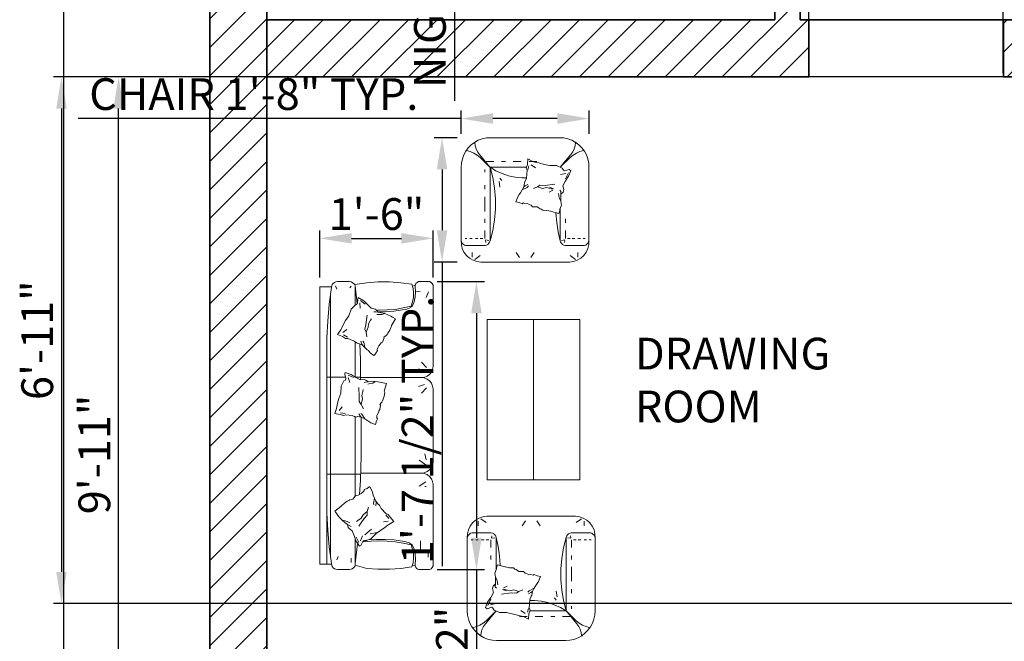
# Model space of a CAD drawing. Units: inches. Extents: x -33 to 381, y -443 to 47.
# Tile 2 of 5: x -33 to 122, y -308 to -210. Entities that reach past the tile are written whole.
import ezdxf

# ---------------------------------------------------------------- set-up
doc = ezdxf.new("R2010")
doc.units = ezdxf.units.IN
for name, color, linetype, lineweight in [('A-ANNO-DIMS', 2, 'Continuous', 18), ('A-AREA-IDEN', 7, 'Continuous', 18), ('A-WALL', 7, 'Continuous', 35), ('A-WALL-PATT', 251, 'Continuous', 13), ('furn', 8, 'Continuous', 13)]:
    doc.layers.add(name, color=color, linetype=linetype, lineweight=lineweight)
doc.styles.get("Standard").update_dxf_attribs({"font": 'arial.ttf'})
doc.dimstyles.new('ISO-25', dxfattribs={"dimtxt": 5, "dimasz": 5, "dimexe": 1.25, "dimexo": 0.625, "dimtad": 1, "dimlunit": 3, "dimtxsty": 'Standard', "dimcen": 2.5, "dimadec": 0, "dimazin": 0, "dimtfac": 1, "dimtmove": 0, "dimatfit": 3, "dimfxl": 1, "dimarcsym": 0})

# ---------------------------------------------------------------- blocks, each defined once
blk = doc.blocks.new('sofa-43')
at = {"color": 0, "linetype": 'ByBlock'}
for p, q in [((-0.038, 0.929), (-0.045, 0.917)), ((-0.045, 0.917), (-0.038, 0.929)), ((-0.045, 0.917), (-0.045, 0.824)), ((-0.045, 0.917), (-0.045, 0.824)), ((-0.028, 0.939), (-0.038, 0.929)), ((-0.038, 0.929), (-0.028, 0.939)), ((-0.015, 0.947), (-0.028, 0.939)), ((-0.028, 0.939), (-0.015, 0.947)), ((-0.003, 0.947), (-0.015, 0.947)), ((-0.015, 0.947), (-0.003, 0.947)), ((0.665, 0.947), (-0.003, 0.947)), ((-0.003, 0.947), (0.665, 0.947)), ((0.042, 0.909), (0.087, 0.889)), ((0.687, 0.942), (0.665, 0.947)), ((0.687, 0.942), (0.665, 0.947)), ((0.712, 0.932), (0.687, 0.942)), ((0.712, 0.932), (0.687, 0.942)), ((0.73, 0.917), (0.712, 0.932)), ((0.73, 0.917), (0.712, 0.932)), ((0.745, 0.897), (0.73, 0.917)), ((0.745, 0.897), (0.73, 0.917)), ((0.785, 0.917), (0.77, 0.897)), ((0.77, 0.897), (0.785, 0.917)), ((0.802, 0.932), (0.785, 0.917)), ((0.785, 0.917), (0.802, 0.932)), ((0.827, 0.942), (0.802, 0.932)), ((0.802, 0.932), (0.827, 0.942)), ((0.85, 0.947), (0.827, 0.942)), ((0.827, 0.942), (0.85, 0.947)), ((1.462, 0.947), (0.85, 0.947)), ((0.85, 0.947), (1.462, 0.947)), ((1.487, 0.942), (1.462, 0.947)), ((1.487, 0.942), (1.462, 0.947)), ((1.509, 0.932), (1.487, 0.942)), ((1.509, 0.932), (1.487, 0.942)), ((1.527, 0.917), (1.509, 0.932)), ((1.527, 0.917), (1.509, 0.932)), ((1.542, 0.897), (1.527, 0.917)), ((1.542, 0.897), (1.527, 0.917)), ((1.582, 0.917), (1.567, 0.897)), ((1.567, 0.897), (1.582, 0.917)), ((1.602, 0.932), (1.582, 0.917)), ((1.582, 0.917), (1.602, 0.932)), ((1.624, 0.942), (1.602, 0.932)), ((1.602, 0.932), (1.624, 0.942)), ((1.647, 0.947), (1.624, 0.942)), ((1.624, 0.942), (1.647, 0.947)), ((2.317, 0.947), (1.647, 0.947)), ((1.647, 0.947), (2.317, 0.947)), ((2.257, 0.904), (2.207, 0.904)), ((2.329, 0.947), (2.317, 0.947)), ((2.329, 0.947), (2.317, 0.947)), ((2.342, 0.939), (2.329, 0.947)), ((2.342, 0.939), (2.329, 0.947)), ((2.352, 0.929), (2.342, 0.939)), ((2.352, 0.929), (2.342, 0.939)), ((2.359, 0.917), (2.352, 0.929)), ((2.359, 0.917), (2.352, 0.929)), ((2.359, 0.824), (2.359, 0.917)), ((2.359, 0.917), (2.359, 0.824)), ((-0.045, 0.824), (-0.038, 0.812)), ((-0.045, 0.824), (-0.038, 0.812)), ((0.04, 0.799), (0.037, 0.839)), ((0.672, 0.892), (0.627, 0.849)), ((0.7, 0.874), (0.685, 0.824)), ((0.755, 0.872), (0.745, 0.897)), ((0.755, 0.872), (0.745, 0.897)), ((0.757, 0.849), (0.755, 0.872)), ((0.757, 0.849), (0.755, 0.872)), ((0.76, 0.872), (0.757, 0.849)), ((0.757, 0.849), (0.76, 0.872)), ((0.757, 0.345), (0.757, 0.849)), ((0.77, 0.897), (0.76, 0.872)), ((0.76, 0.872), (0.77, 0.897)), ((0.815, 0.874), (0.83, 0.824)), ((0.842, 0.892), (0.887, 0.849)), ((1.442, 0.887), (1.394, 0.877)), ((1.484, 0.884), (1.447, 0.829)), ((1.552, 0.872), (1.542, 0.897)), ((1.552, 0.872), (1.542, 0.897)), ((1.554, 0.849), (1.552, 0.872)), ((1.554, 0.849), (1.552, 0.872)), ((1.557, 0.872), (1.554, 0.849)), ((1.554, 0.849), (1.557, 0.872)), ((1.554, 0.345), (1.554, 0.849)), ((1.567, 0.897), (1.557, 0.872)), ((1.557, 0.872), (1.567, 0.897)), ((1.627, 0.884), (1.664, 0.829)), ((1.667, 0.887), (1.667, 0.877)), ((2.194, 0.842), (2.119, 0.842)), ((2.352, 0.812), (2.359, 0.824)), ((2.359, 0.824), (2.352, 0.812)), ((-0.038, 0.812), (-0.028, 0.802)), ((-0.038, 0.812), (-0.028, 0.802)), ((-0.023, 0.769), (-0.035, 0.677)), ((-0.023, 0.769), (-0.035, 0.677)), ((-0.028, 0.802), (-0.015, 0.797)), ((-0.028, 0.802), (-0.015, 0.797)), ((0.012, 0.779), (-0.023, 0.769)), ((-0.0064, 0.7737), (-0.023, 0.769)), ((-0.015, 0.797), (-0.0064, 0.7737)), ((-0.015, 0.797), (-0.003, 0.797)), ((-0.0064, 0.7737), (-0.015, 0.797)), ((0.04, 0.799), (-0.003, 0.797)), ((0.05, 0.782), (0.012, 0.779)), ((0.082, 0.797), (0.04, 0.799)), ((0.087, 0.782), (0.05, 0.782)), ((0.125, 0.787), (0.082, 0.797)), ((0.125, 0.774), (0.087, 0.782)), ((0.162, 0.772), (0.125, 0.787)), ((0.16, 0.762), (0.125, 0.774)), ((0.175, 0.697), (0.16, 0.762)), ((0.177, 0.747), (0.162, 0.772)), ((0.187, 0.719), (0.177, 0.747)), ((2.127, 0.719), (2.137, 0.747)), ((2.137, 0.747), (2.152, 0.772)), ((2.139, 0.697), (2.154, 0.762)), ((2.152, 0.772), (2.189, 0.787)), ((2.154, 0.762), (2.189, 0.774)), ((2.189, 0.787), (2.232, 0.797)), ((2.189, 0.774), (2.227, 0.782)), ((2.227, 0.782), (2.264, 0.782)), ((2.232, 0.797), (2.274, 0.799)), ((2.264, 0.782), (2.302, 0.779)), ((2.274, 0.799), (2.317, 0.797)), ((2.302, 0.779), (2.337, 0.769)), ((2.329, 0.797), (2.317, 0.797)), ((2.3218, 0.7734), (2.329, 0.797)), ((2.3218, 0.7734), (2.329, 0.797)), ((2.337, 0.769), (2.3218, 0.7734)), ((2.329, 0.797), (2.342, 0.802)), ((2.342, 0.802), (2.329, 0.797)), ((2.349, 0.677), (2.337, 0.769)), ((2.337, 0.769), (2.349, 0.677)), ((2.342, 0.802), (2.352, 0.812)), ((2.352, 0.812), (2.342, 0.802)), ((-0.035, 0.677), (-0.043, 0.582)), ((-0.035, 0.677), (-0.043, 0.582)), ((0.187, 0.629), (0.175, 0.697)), ((0.192, 0.692), (0.187, 0.719)), ((0.202, 0.619), (0.192, 0.692)), ((2.112, 0.619), (2.122, 0.692)), ((2.122, 0.692), (2.127, 0.719)), ((2.127, 0.629), (2.139, 0.697)), ((2.357, 0.582), (2.349, 0.677)), ((2.349, 0.677), (2.357, 0.582)), ((-0.043, 0.582), (-0.043, 0.484)), ((-0.043, 0.582), (-0.043, 0.484)), ((0.192, 0.562), (0.187, 0.629)), ((0.207, 0.547), (0.202, 0.619)), ((0.245, 0.594), (0.232, 0.567)), ((0.252, 0.607), (0.245, 0.594)), ((0.267, 0.632), (0.252, 0.607)), ((0.322, 0.599), (0.267, 0.632)), ((0.332, 0.597), (0.322, 0.599)), ((0.362, 0.584), (0.332, 0.597)), ((0.385, 0.569), (0.362, 0.584)), ((1.922, 0.587), (1.899, 0.572)), ((1.934, 0.577), (1.902, 0.552)), ((1.957, 0.617), (1.922, 0.587)), ((1.982, 0.577), (1.957, 0.617)), ((1.989, 0.567), (1.982, 0.577)), ((2.107, 0.547), (2.112, 0.619)), ((2.122, 0.562), (2.127, 0.629)), ((2.357, 0.484), (2.357, 0.582)), ((2.357, 0.582), (2.357, 0.484)), ((0.195, 0.497), (0.192, 0.562)), ((0.195, 0.482), (0.195, 0.497)), ((0.207, 0.492), (0.207, 0.547)), ((0.215, 0.514), (0.212, 0.487)), ((0.222, 0.542), (0.215, 0.514)), ((0.232, 0.567), (0.222, 0.542)), ((0.222, 0.542), (0.23, 0.519)), ((0.23, 0.519), (0.23, 0.497)), ((0.23, 0.497), (0.23, 0.477)), ((0.397, 0.562), (0.385, 0.569)), ((0.405, 0.554), (0.397, 0.562)), ((0.42, 0.534), (0.405, 0.554)), ((0.425, 0.537), (0.42, 0.534)), ((0.46, 0.524), (0.425, 0.537)), ((0.467, 0.512), (0.46, 0.524)), ((0.475, 0.507), (0.467, 0.512)), ((0.492, 0.492), (0.475, 0.507)), ((0.797, 0.517), (0.792, 0.484)), ((0.8, 0.529), (0.797, 0.517)), ((0.807, 0.557), (0.8, 0.529)), ((0.87, 0.539), (0.807, 0.557)), ((0.88, 0.542), (0.87, 0.539)), ((0.912, 0.537), (0.88, 0.542)), ((0.937, 0.529), (0.912, 0.537)), ((0.952, 0.524), (0.937, 0.529)), ((0.962, 0.519), (0.952, 0.524)), ((0.982, 0.502), (0.962, 0.519)), ((0.987, 0.507), (0.982, 0.502)), ((1.022, 0.502), (0.987, 0.507)), ((1.035, 0.492), (1.022, 0.502)), ((1.822, 0.499), (1.814, 0.487)), ((1.849, 0.514), (1.822, 0.499)), ((1.827, 0.504), (1.832, 0.502)), ((1.892, 0.552), (1.849, 0.514)), ((1.899, 0.572), (1.892, 0.552)), ((1.954, 0.572), (1.962, 0.532)), ((2.009, 0.542), (1.989, 0.567)), ((2.034, 0.507), (2.009, 0.542)), ((2.057, 0.47), (2.034, 0.507)), ((2.107, 0.474), (2.107, 0.547)), ((2.119, 0.497), (2.122, 0.562)), ((2.122, 0.43), (2.119, 0.497)), ((-0.043, 0.484), (-0.035, 0.392)), ((-0.043, 0.484), (-0.035, 0.392)), ((0.177, 0.43), (0.145, 0.395)), ((0.185, 0.462), (0.177, 0.43)), ((0.192, 0.472), (0.185, 0.462)), ((0.212, 0.487), (0.192, 0.472)), ((0.207, 0.467), (0.212, 0.487)), ((0.207, 0.452), (0.207, 0.467)), ((0.277, 0.425), (0.265, 0.432)), ((0.307, 0.407), (0.277, 0.425)), ((0.507, 0.484), (0.492, 0.492)), ((0.522, 0.479), (0.507, 0.484)), ((0.532, 0.482), (0.522, 0.479)), ((0.552, 0.467), (0.532, 0.482)), ((0.532, 0.407), (0.55, 0.422)), ((0.55, 0.422), (0.572, 0.452)), ((0.57, 0.457), (0.552, 0.467)), ((0.572, 0.452), (0.57, 0.457)), ((0.79, 0.462), (0.787, 0.432)), ((0.787, 0.432), (0.792, 0.407)), ((0.792, 0.484), (0.79, 0.462)), ((0.79, 0.462), (0.802, 0.442)), ((0.802, 0.442), (0.807, 0.42)), ((0.807, 0.42), (0.812, 0.4)), ((1.042, 0.492), (1.035, 0.492)), ((1.062, 0.482), (1.042, 0.492)), ((1.074, 0.477), (1.062, 0.482)), ((1.092, 0.477), (1.074, 0.477)), ((1.102, 0.482), (1.092, 0.477)), ((1.124, 0.472), (1.102, 0.482)), ((1.122, 0.41), (1.134, 0.427)), ((1.144, 0.467), (1.124, 0.472)), ((1.134, 0.427), (1.147, 0.465)), ((1.147, 0.465), (1.144, 0.467)), ((1.704, 0.437), (1.669, 0.417)), ((1.669, 0.417), (1.669, 0.412)), ((1.669, 0.412), (1.682, 0.395)), ((1.724, 0.442), (1.704, 0.437)), ((1.737, 0.447), (1.724, 0.442)), ((1.762, 0.457), (1.737, 0.447)), ((1.789, 0.467), (1.762, 0.457)), ((1.762, 0.457), (1.807, 0.45)), ((1.814, 0.487), (1.789, 0.467)), ((1.789, 0.467), (1.802, 0.47)), ((1.802, 0.47), (1.827, 0.467)), ((1.807, 0.45), (1.819, 0.452)), ((2.069, 0.377), (2.022, 0.432)), ((2.062, 0.422), (2.049, 0.479)), ((2.102, 0.427), (2.057, 0.47)), ((2.119, 0.382), (2.102, 0.427)), ((2.112, 0.405), (2.107, 0.474)), ((2.127, 0.362), (2.122, 0.43)), ((2.349, 0.392), (2.357, 0.484)), ((2.357, 0.484), (2.349, 0.392)), ((-0.035, 0.392), (-0.02, 0.292)), ((-0.035, 0.392), (-0.02, 0.292)), ((0.117, 0.367), (0.087, 0.322)), ((0.112, 0.34), (0.145, 0.38)), ((0.145, 0.395), (0.117, 0.367)), ((0.132, 0.335), (0.177, 0.337)), ((0.237, 0.397), (0.315, 0.385)), ((0.337, 0.405), (0.307, 0.407)), ((0.315, 0.385), (0.352, 0.375)), ((0.377, 0.387), (0.337, 0.405)), ((0.352, 0.375), (0.377, 0.387)), ((0.377, 0.387), (0.417, 0.392)), ((0.462, 0.367), (0.452, 0.36)), ((0.477, 0.35), (0.452, 0.342)), ((0.505, 0.377), (0.462, 0.367)), ((0.472, 0.327), (0.485, 0.357)), ((0.607, 0.34), (0.475, 0.335)), ((0.485, 0.357), (0.477, 0.35)), ((0.485, 0.357), (0.505, 0.377)), ((0.505, 0.377), (0.525, 0.397)), ((0.525, 0.397), (0.532, 0.407)), ((0.775, 0.34), (0.607, 0.34)), ((0.775, 0.34), (0.752, 0.297)), ((0.752, 0.297), (0.752, 0.34)), ((0.777, 0.385), (0.772, 0.372)), ((0.772, 0.372), (0.775, 0.34)), ((0.792, 0.407), (0.777, 0.385)), ((0.795, 0.382), (0.792, 0.407)), ((0.797, 0.37), (0.795, 0.382)), ((0.84, 0.325), (0.917, 0.33)), ((0.872, 0.36), (0.857, 0.362)), ((0.905, 0.35), (0.872, 0.36)), ((0.935, 0.357), (0.905, 0.35)), ((0.917, 0.33), (0.957, 0.33)), ((0.98, 0.347), (0.935, 0.357)), ((0.957, 0.33), (0.98, 0.347)), ((0.98, 0.347), (1.017, 0.365)), ((1.062, 0.352), (1.057, 0.342)), ((1.082, 0.34), (1.059, 0.327)), ((1.102, 0.375), (1.062, 0.352)), ((1.087, 0.347), (1.082, 0.34)), ((1.082, 0.317), (1.087, 0.347)), ((1.087, 0.347), (1.102, 0.375)), ((1.409, 0.347), (1.087, 0.347)), ((1.102, 0.375), (1.117, 0.4)), ((1.117, 0.4), (1.122, 0.41)), ((1.612, 0.34), (1.409, 0.347)), ((1.562, 0.06), (1.562, 0.34)), ((1.732, 0.332), (1.612, 0.34)), ((1.682, 0.395), (1.692, 0.372)), ((1.692, 0.372), (1.702, 0.372)), ((1.702, 0.372), (1.714, 0.36)), ((1.714, 0.36), (1.724, 0.347)), ((1.724, 0.347), (1.734, 0.325)), ((1.874, 0.397), (1.837, 0.407)), ((1.874, 0.397), (1.902, 0.362)), ((1.904, 0.397), (1.874, 0.397)), ((1.902, 0.362), (1.929, 0.347)), ((1.932, 0.372), (1.904, 0.397)), ((1.929, 0.347), (1.949, 0.317)), ((1.997, 0.325), (1.932, 0.372)), ((2.119, 0.34), (2.077, 0.357)), ((2.117, 0.375), (2.112, 0.405)), ((2.117, 0.37), (2.119, 0.382)), ((2.124, 0.36), (2.117, 0.37)), ((2.119, 0.302), (2.164, 0.332)), ((2.157, 0.342), (2.124, 0.36)), ((2.129, 0.357), (2.127, 0.362)), ((2.164, 0.332), (2.157, 0.342)), ((2.322, 0.297), (2.349, 0.392)), ((2.349, 0.392), (2.322, 0.297)), ((-0.043, 0.262), (-0.045, 0.247)), ((-0.043, 0.262), (-0.045, 0.247)), ((-0.045, 0.247), (-0.045, 0.147)), ((-0.045, 0.247), (-0.045, 0.147)), ((-0.038, 0.272), (-0.043, 0.262)), ((-0.038, 0.272), (-0.043, 0.262)), ((-0.03, 0.282), (-0.038, 0.272)), ((-0.03, 0.282), (-0.038, 0.272)), ((-0.02, 0.292), (-0.03, 0.282)), ((-0.02, 0.292), (-0.03, 0.282)), ((-0.008, 0.297), (-0.02, 0.292)), ((0.14, 0.312), (-0.008, 0.297)), ((-0.008, 0.297), (0.15, 0.297)), ((0.005, 0.297), (-0.008, 0.297)), ((-0.005, 0.262), (0.007, 0.25)), ((0.087, 0.322), (0.1, 0.317)), ((0.1, 0.317), (0.135, 0.315)), ((0.135, 0.315), (0.147, 0.307)), ((0.147, 0.307), (0.152, 0.295)), ((0.152, 0.295), (0.185, 0.262)), ((0.185, 0.262), (0.242, 0.242)), ((0.43, 0.235), (0.452, 0.287)), ((0.452, 0.287), (0.47, 0.312)), ((0.46, 0.297), (0.752, 0.297)), ((0.467, 0.307), (0.462, 0.307)), ((0.47, 0.312), (0.472, 0.327)), ((0.732, 0.262), (0.715, 0.212)), ((0.752, 0.297), (0.732, 0.262)), ((0.737, 0.237), (0.755, 0.282)), ((0.755, 0.237), (0.797, 0.25)), ((1.067, 0.217), (1.074, 0.272)), ((1.074, 0.272), (1.087, 0.302)), ((1.084, 0.297), (1.079, 0.292)), ((1.087, 0.302), (1.082, 0.317)), ((1.0855, 0.2985), (1.084, 0.297)), ((1.084, 0.297), (1.0848, 0.297)), ((1.084, 0.297), (1.562, 0.297)), ((1.0848, 0.297), (1.0855, 0.2985)), ((1.562, 0.297), (1.747, 0.297)), ((1.734, 0.325), (1.737, 0.32)), ((1.737, 0.32), (1.742, 0.302)), ((1.742, 0.302), (1.767, 0.28)), ((1.767, 0.28), (1.772, 0.28)), ((1.772, 0.28), (1.777, 0.252)), ((1.777, 0.252), (1.782, 0.242)), ((1.949, 0.317), (1.957, 0.307)), ((1.959, 0.23), (1.969, 0.25)), ((1.994, 0.25), (1.982, 0.232)), ((1.999, 0.262), (1.994, 0.25)), ((2.017, 0.245), (2.037, 0.272)), ((2.037, 0.272), (2.082, 0.29)), ((2.082, 0.29), (2.119, 0.302)), ((2.134, 0.327), (2.089, 0.305)), ((2.104, 0.297), (2.309, 0.297)), ((2.117, 0.317), (2.114, 0.317)), ((2.144, 0.315), (2.137, 0.317)), ((2.137, 0.315), (2.137, 0.317)), ((2.309, 0.297), (2.144, 0.315)), ((2.299, 0.262), (2.264, 0.262)), ((2.322, 0.297), (2.309, 0.297)), ((2.334, 0.292), (2.322, 0.297)), ((2.334, 0.292), (2.322, 0.297)), ((2.344, 0.282), (2.334, 0.292)), ((2.344, 0.282), (2.334, 0.292)), ((2.352, 0.272), (2.344, 0.282)), ((2.352, 0.272), (2.344, 0.282)), ((2.357, 0.262), (2.352, 0.272)), ((2.357, 0.262), (2.352, 0.272)), ((2.359, 0.247), (2.357, 0.262)), ((2.359, 0.247), (2.357, 0.262)), ((2.359, 0.147), (2.359, 0.247)), ((2.359, 0.147), (2.359, 0.247)), ((0.242, 0.242), (0.28, 0.215)), ((0.28, 0.215), (0.317, 0.195)), ((0.317, 0.195), (0.347, 0.182)), ((0.347, 0.182), (0.357, 0.175)), ((0.38, 0.192), (0.355, 0.225)), ((0.357, 0.175), (0.397, 0.147)), ((0.397, 0.147), (0.415, 0.19)), ((0.4, 0.197), (0.42, 0.232)), ((0.415, 0.19), (0.43, 0.215)), ((0.43, 0.215), (0.43, 0.235)), ((0.715, 0.212), (0.727, 0.21)), ((0.727, 0.21), (0.765, 0.217)), ((0.752, 0.06), (0.752, 0.215)), ((0.765, 0.217), (0.777, 0.215)), ((0.777, 0.215), (0.785, 0.202)), ((0.785, 0.202), (0.827, 0.18)), ((0.827, 0.18), (0.887, 0.175)), ((0.887, 0.175), (0.93, 0.16)), ((1.032, 0.162), (1, 0.187)), ((1.05, 0.172), (1.057, 0.212)), ((1.057, 0.125), (1.064, 0.17)), ((1.064, 0.17), (1.072, 0.197)), ((1.072, 0.197), (1.067, 0.217)), ((1.782, 0.242), (1.789, 0.23)), ((1.789, 0.23), (1.804, 0.207)), ((1.804, 0.207), (1.827, 0.182)), ((1.827, 0.182), (1.834, 0.177)), ((1.834, 0.177), (1.872, 0.125)), ((1.907, 0.15), (1.929, 0.17)), ((1.929, 0.17), (1.947, 0.187)), ((1.947, 0.187), (1.952, 0.212)), ((1.947, 0.187), (1.967, 0.21)), ((1.952, 0.212), (1.959, 0.23)), ((1.967, 0.21), (1.982, 0.232)), ((1.982, 0.232), (2.007, 0.237)), ((2.007, 0.237), (2.017, 0.245)), ((-0.045, 0.147), (-0.043, 0.135)), ((-0.045, 0.147), (-0.043, 0.135)), ((-0.043, 0.135), (-0.038, 0.122)), ((-0.043, 0.135), (-0.038, 0.122)), ((-0.038, 0.122), (-0.03, 0.112)), ((-0.038, 0.122), (-0.03, 0.112)), ((-0.03, 0.112), (-0.02, 0.105)), ((-0.03, 0.112), (-0.02, 0.105)), ((-0.02, 0.105), (-0.008, 0.1)), ((-0.02, 0.105), (-0.008, 0.1)), ((-0.008, 0.132), (0.02, 0.142)), ((-0.008, 0.1), (0, 0.0982)), ((-0.008, 0.1), (0.005, 0.097)), ((0, 0.1), (0, 0)), ((0, 0.0982), (0, 0)), ((0.005, 0.097), (0.145, 0.08)), ((0.072, 0.09), (0.752, 0.09)), ((0.752, 0.09), (1.562, 0.09)), ((0.93, 0.16), (0.97, 0.147)), ((0.97, 0.147), (1.002, 0.142)), ((1.002, 0.142), (1.015, 0.14)), ((1.015, 0.14), (1.057, 0.125)), ((1.562, 0.09), (2.242, 0.09)), ((1.872, 0.125), (1.894, 0.142)), ((1.894, 0.142), (1.907, 0.15)), ((2.169, 0.08), (2.309, 0.097)), ((2.277, 0.142), (2.249, 0.155)), ((2.309, 0.097), (2.322, 0.1)), ((2.314, 0.0982), (2.322, 0.1)), ((2.314, 0.1), (2.314, 0)), ((2.314, 0), (2.314, 0.0982)), ((2.322, 0.1), (2.334, 0.105)), ((2.322, 0.1), (2.334, 0.105)), ((2.334, 0.105), (2.344, 0.112)), ((2.334, 0.105), (2.344, 0.112)), ((2.344, 0.112), (2.352, 0.122)), ((2.344, 0.112), (2.352, 0.122)), ((2.352, 0.122), (2.357, 0.135)), ((2.352, 0.122), (2.357, 0.135)), ((2.357, 0.135), (2.359, 0.147)), ((2.357, 0.135), (2.359, 0.147)), ((0, 0), (2.314, 0)), ((0, 0), (2.314, 0)), ((0.145, 0.08), (0.285, 0.067)), ((0.285, 0.067), (0.425, 0.06)), ((0.425, 0.06), (2.314, 0.06)), ((1.889, 0.06), (2.029, 0.067)), ((2.029, 0.067), (2.169, 0.08))]:
    blk.add_line(p, q, dxfattribs=at)
blk = doc.blocks.new('sofa-38')
at = {"color": 0, "linetype": 'ByBlock'}
for p, q in [((-0.1449, 0.828), (-0.1656, 0.81)), ((-0.1449, 0.828), (-0.1656, 0.81)), ((-0.1206, 0.8424), (-0.1449, 0.828)), ((-0.1206, 0.8424), (-0.1449, 0.828)), ((-0.126, 0.8208), (-0.126, 0.7884)), ((-0.0945, 0.8514), (-0.1206, 0.8424)), ((-0.0945, 0.8514), (-0.1206, 0.8424)), ((-0.072, 0.8109), (-0.108, 0.8379)), ((-0.0666, 0.855), (-0.0945, 0.8514)), ((-0.0666, 0.855), (-0.0945, 0.8514)), ((0.2376, 0.855), (-0.0666, 0.855)), ((0.2376, 0.855), (-0.0666, 0.855)), ((0.1764, 0.7884), (0.198, 0.8235)), ((0.5418, 0.855), (0.2376, 0.855)), ((0.5418, 0.855), (0.2376, 0.855)), ((0.2772, 0.8235), (0.2988, 0.7884)), ((0.5697, 0.8514), (0.5418, 0.855)), ((0.5697, 0.8514), (0.5418, 0.855)), ((0.5472, 0.8109), (0.5832, 0.8379)), ((0.5958, 0.8424), (0.5697, 0.8514)), ((0.5958, 0.8424), (0.5697, 0.8514)), ((0.6201, 0.828), (0.5958, 0.8424)), ((0.6201, 0.828), (0.5958, 0.8424)), ((0.6012, 0.8208), (0.6012, 0.7884)), ((0.6408, 0.81), (0.6201, 0.828)), ((0.6408, 0.81), (0.6201, 0.828)), ((-0.1944, 0.7614), (-0.2007, 0.7344)), ((-0.1944, 0.7614), (-0.2007, 0.7344)), ((-0.1827, 0.7875), (-0.1944, 0.7614)), ((-0.1827, 0.7875), (-0.1944, 0.7614)), ((-0.1656, 0.81), (-0.1827, 0.7875)), ((-0.1656, 0.81), (-0.1827, 0.7875)), ((0.6579, 0.7875), (0.6408, 0.81)), ((0.6579, 0.7875), (0.6408, 0.81)), ((0.6696, 0.7614), (0.6579, 0.7875)), ((0.6696, 0.7614), (0.6579, 0.7875)), ((0.6759, 0.7344), (0.6696, 0.7614)), ((0.6759, 0.7344), (0.6696, 0.7614)), ((-0.2007, 0.7344), (-0.2016, 0.7065)), ((-0.2007, 0.7344), (-0.2016, 0.7065)), ((-0.2016, 0.7065), (-0.1989, 0.7164)), ((-0.2016, 0.7065), (-0.2016, 0.2034)), ((-0.2016, 0.2034), (-0.2016, 0.7065)), ((-0.1989, 0.7164), (-0.1944, 0.7254)), ((-0.1944, 0.7254), (-0.1872, 0.7326)), ((-0.1872, 0.7326), (-0.1791, 0.738)), ((-0.1791, 0.738), (-0.1692, 0.7407)), ((-0.1746, 0.693), (-0.162, 0.693)), ((-0.1692, 0.7407), (-0.1593, 0.7416)), ((-0.1593, 0.7416), (-0.0486, 0.7416)), ((-0.1431, 0.693), (-0.126, 0.693)), ((-0.1035, 0.693), (-0.0864, 0.693)), ((-0.072, 0.693), (-0.054, 0.693)), ((-0.0486, 0.7416), (-0.0378, 0.7416)), ((-0.0396, 0.693), (-0.0396, 0.639)), ((-0.0378, 0.7416), (-0.0279, 0.7389)), ((-0.0351, 0.7074), (-0.0324, 0.72)), ((-0.0351, 0.7029), (-0.0126, 0.7074)), ((-0.0279, 0.7389), (-0.0189, 0.7335)), ((-0.0189, 0.7335), (-0.0117, 0.7263)), ((-0.0117, 0.7263), (-0.0063, 0.7182)), ((-0.0063, 0.7182), (-0.0027, 0.7083)), ((0.0099, 0.6462), (-0.0027, 0.7083)), ((-0.0027, 0.7083), (-0.0027, 0.6975)), ((-0.0027, 0.6975), (-0.0027, 0.489)), ((0.4779, 0.7083), (0.4599, 0.6372)), ((0.4779, 0.7083), (0.4815, 0.7182)), ((0.4779, 0.6975), (0.4779, 0.7083)), ((0.4779, 0.2034), (0.4779, 0.6975)), ((0.4815, 0.7182), (0.4869, 0.7263)), ((0.4869, 0.7263), (0.4941, 0.7335)), ((0.5103, 0.7029), (0.4878, 0.7074)), ((0.4941, 0.7335), (0.5031, 0.7389)), ((0.5031, 0.7389), (0.513, 0.7416)), ((0.5103, 0.7074), (0.5076, 0.72)), ((0.513, 0.7416), (0.5238, 0.7416)), ((0.5148, 0.693), (0.5148, 0.639)), ((0.5238, 0.7416), (0.6345, 0.7416)), ((0.5472, 0.693), (0.5292, 0.693)), ((0.5787, 0.693), (0.5616, 0.693)), ((0.6183, 0.693), (0.6012, 0.693)), ((0.6345, 0.7416), (0.6444, 0.7407)), ((0.6498, 0.693), (0.6372, 0.693)), ((0.6444, 0.7407), (0.6543, 0.738)), ((0.6543, 0.738), (0.6624, 0.7326)), ((0.6624, 0.7326), (0.6696, 0.7254)), ((0.6696, 0.7254), (0.6741, 0.7164)), ((0.6741, 0.7164), (0.6768, 0.7065)), ((0.6768, 0.7065), (0.6759, 0.7344)), ((0.6768, 0.7065), (0.6759, 0.7344)), ((0.6768, 0.2034), (0.6768, 0.7065)), ((0.6768, 0.7065), (0.6768, 0.2034)), ((0.0198, 0.5832), (0.0099, 0.6462)), ((0.4599, 0.6372), (0.4473, 0.5652)), ((-0.0396, 0.585), (-0.0396, 0.558)), ((0.0252, 0.5193), (0.0198, 0.5832)), ((0.4473, 0.5652), (0.441, 0.4923)), ((0.5148, 0.585), (0.5148, 0.558)), ((-0.0014, 0.4925), (-0.0124, 0.4628)), ((-0.0003, 0.5002), (-0.0014, 0.4925)), ((0.0063, 0.5211), (-0.0003, 0.5002)), ((0.0558, 0.5068), (0.0063, 0.5211)), ((0.0253, 0.5155), (0.0252, 0.5193)), ((0.0602, 0.5057), (0.0558, 0.5068)), ((0.0877, 0.5002), (0.0602, 0.5057)), ((0.1163, 0.4991), (0.0877, 0.5002)), ((0.1262, 0.4903), (0.1163, 0.4991)), ((0.1339, 0.4892), (0.1262, 0.4903)), ((0.1537, 0.4749), (0.1339, 0.4892)), ((0.1537, 0.4749), (0.1537, 0.4749)), ((0.1856, 0.4749), (0.1537, 0.4749)), ((0.1966, 0.4639), (0.1856, 0.4749)), ((0.441, 0.4923), (0.441, 0.4194)), ((0.5148, 0.4077), (0.5148, 0.5067)), ((-0.0124, 0.4628), (-0.008, 0.4364)), ((-0.008, 0.4364), (-0.008, 0.4133)), ((-0.008, 0.4364), (0.0019, 0.4188)), ((-0.008, 0.4133), (-0.008, 0.3891)), ((0.0019, 0.4188), (0.0052, 0.4001)), ((0.2054, 0.4617), (0.1966, 0.4639)), ((0.2219, 0.4518), (0.2054, 0.4617)), ((0.2351, 0.4551), (0.2219, 0.4518)), ((0.2505, 0.4485), (0.2351, 0.4551)), ((0.2582, 0.454), (0.2505, 0.4485)), ((0.278, 0.4452), (0.2582, 0.454)), ((0.3011, 0.4408), (0.278, 0.4452)), ((0.278, 0.3913), (0.2868, 0.4067)), ((0.2868, 0.4067), (0.3011, 0.4408)), ((0.3011, 0.4408), (0.3011, 0.4408)), ((0.441, 0.4194), (0.4473, 0.3465)), ((-0.0289, 0.3572), (-0.0245, 0.3737)), ((-0.0223, 0.3308), (-0.0289, 0.3572)), ((-0.0245, 0.3737), (-0.008, 0.3891)), ((-0.008, 0.3891), (-0.0091, 0.3704)), ((-0.0091, 0.3704), (-0.0014, 0.3605)), ((0.0052, 0.4001), (0.0085, 0.3836)), ((0.0415, 0.3506), (0.069, 0.3407)), ((0.047, 0.3616), (0.0723, 0.3748)), ((0.0591, 0.3517), (0.0503, 0.3528)), ((0.0899, 0.3429), (0.0591, 0.3517)), ((0.1174, 0.3484), (0.0899, 0.3429)), ((0.1526, 0.3374), (0.1174, 0.3484)), ((0.1526, 0.3374), (0.1801, 0.3484)), ((0.2153, 0.3319), (0.2241, 0.3418)), ((0.2241, 0.3418), (0.2571, 0.3594)), ((0.2571, 0.3594), (0.2472, 0.3374)), ((0.2571, 0.3594), (0.2703, 0.3792)), ((0.2703, 0.3792), (0.278, 0.3913)), ((0.4167, 0.3015), (0.4104, 0.3402)), ((0.4473, 0.3465), (0.4599, 0.2745)), ((0.5148, 0.3267), (0.5148, 0.3537)), ((-0.0619, 0.2648), (-0.041, 0.2956)), ((-0.0597, 0.2417), (-0.041, 0.2835)), ((-0.041, 0.2956), (-0.0223, 0.3308)), ((0.0327, 0.3187), (0.0998, 0.3275)), ((0.0998, 0.3275), (0.1361, 0.3253)), ((0.1361, 0.3253), (0.1526, 0.3374)), ((0.2362, 0.3308), (0.2186, 0.3209)), ((0.2285, 0.2791), (0.223, 0.2241)), ((0.261, 0.2763), (0.2282, 0.2763)), ((0.2384, 0.3044), (0.2285, 0.2791)), ((0.2472, 0.3374), (0.2362, 0.3308)), ((0.2428, 0.311), (0.2384, 0.3044)), ((0.2472, 0.3374), (0.2428, 0.311)), ((0.3069, 0.2718), (0.261, 0.2763)), ((0.3519, 0.2619), (0.3069, 0.2718)), ((0.4104, 0.2781), (0.3969, 0.2934)), ((0.4599, 0.2745), (0.4779, 0.2034)), ((-0.2016, 0.2034), (-0.1998, 0.1746)), ((-0.1998, 0.1746), (-0.2016, 0.2034)), ((-0.0762, 0.2274), (-0.0619, 0.2648)), ((-0.0652, 0.2186), (-0.0762, 0.2274)), ((-0.0333, 0.2285), (-0.0652, 0.2186)), ((-0.0432, 0.2461), (-0.0047, 0.2538)), ((-0.0256, 0.223), (-0.0333, 0.2285)), ((-0.0179, 0.2087), (-0.0256, 0.223)), ((0.0206, 0.1922), (-0.0179, 0.2087)), ((0.1966, 0.1856), (0.1669, 0.2065)), ((0.212, 0.1944), (0.2186, 0.2208)), ((0.2307, 0.2098), (0.2219, 0.1845)), ((0.223, 0.2241), (0.2307, 0.2098)), ((0.2285, 0.2034), (0.2376, 0.2034)), ((0.2376, 0.2034), (0.4779, 0.2034)), ((0.396, 0.2466), (0.3519, 0.2619)), ((0.4383, 0.2277), (0.396, 0.2466)), ((0.4779, 0.2034), (0.4383, 0.2277)), ((0.5148, 0.2187), (0.5148, 0.2358)), ((0.675, 0.1746), (0.6768, 0.2034)), ((0.6768, 0.2034), (0.675, 0.1746)), ((-0.1998, 0.1746), (-0.1935, 0.1458)), ((-0.1935, 0.1458), (-0.1998, 0.1746)), ((-0.1935, 0.1458), (-0.1836, 0.1188)), ((-0.1836, 0.1188), (-0.1935, 0.1458)), ((-0.0765, 0.1152), (-0.0045, 0.2016)), ((-0.0045, 0.2016), (-0.0711, 0.135)), ((0.0679, 0.1922), (0.0206, 0.1922)), ((0.0283, 0.19), (0.0283, 0.1911)), ((0.1075, 0.1845), (0.0679, 0.1922)), ((0.1438, 0.1735), (0.1075, 0.1845)), ((0.1702, 0.168), (0.1438, 0.1735)), ((0.1566, 0.1647), (0.2106, 0.1647)), ((0.1845, 0.1647), (0.1702, 0.168)), ((0.2197, 0.146), (0.1845, 0.1647)), ((0.2219, 0.1845), (0.2197, 0.146)), ((0.3186, 0.1647), (0.2646, 0.1647)), ((0.3996, 0.1647), (0.3726, 0.1647)), ((0.5076, 0.1647), (0.4536, 0.1647)), ((0.4797, 0.2016), (0.5517, 0.1152)), ((0.5463, 0.135), (0.4797, 0.2016)), ((0.6588, 0.1188), (0.6687, 0.1458)), ((0.6687, 0.1458), (0.6588, 0.1188)), ((0.6687, 0.1458), (0.675, 0.1746)), ((0.675, 0.1746), (0.6687, 0.1458)), ((-0.1836, 0.1188), (-0.1701, 0.0936)), ((-0.1701, 0.0936), (-0.1836, 0.1188)), ((-0.1701, 0.0936), (-0.153, 0.0702)), ((-0.153, 0.0702), (-0.1701, 0.0936)), ((-0.1395, 0.0954), (-0.1647, 0.0873)), ((-0.153, 0.0702), (-0.1323, 0.0495)), ((-0.1323, 0.0495), (-0.153, 0.0702)), ((-0.1152, 0.1062), (-0.1395, 0.0954)), ((-0.0927, 0.1197), (-0.1152, 0.1062)), ((-0.1062, 0.0558), (-0.0999, 0.0774)), ((-0.0999, 0.0774), (-0.09, 0.0972)), ((-0.0711, 0.135), (-0.0927, 0.1197)), ((-0.09, 0.0972), (-0.0765, 0.1152)), ((0.5679, 0.1197), (0.5463, 0.135)), ((0.5517, 0.1152), (0.5652, 0.0972)), ((0.5652, 0.0972), (0.5751, 0.0774)), ((0.5904, 0.1062), (0.5679, 0.1197)), ((0.5751, 0.0774), (0.5814, 0.0558)), ((0.6147, 0.0954), (0.5904, 0.1062)), ((0.6075, 0.0495), (0.6282, 0.0702)), ((0.6282, 0.0702), (0.6075, 0.0495)), ((0.6399, 0.0873), (0.6147, 0.0954)), ((0.6282, 0.0702), (0.6453, 0.0936)), ((0.6453, 0.0936), (0.6282, 0.0702)), ((0.6453, 0.0936), (0.6588, 0.1188)), ((0.6588, 0.1188), (0.6453, 0.0936)), ((-0.1323, 0.0495), (-0.1082, 0.0312)), ((-0.1098, 0.0324), (-0.1323, 0.0495)), ((-0.0846, 0.018), (-0.1098, 0.0324)), ((-0.1082, 0.0312), (-0.1081, 0.0315)), ((-0.1081, 0.0315), (-0.0846, 0.018)), ((-0.108, 0.0333), (-0.1062, 0.0558)), ((-0.0846, 0.018), (-0.0567, 0.0081)), ((-0.0567, 0.0081), (-0.0846, 0.018)), ((-0.0567, 0.0081), (-0.0288, 0.0018)), ((-0.0288, 0.0018), (-0.0567, 0.0081)), ((-0.0288, 0.0018), (0, 0)), ((0, 0), (-0.0288, 0.0018)), ((0, 0), (0.2376, 0)), ((0.2376, 0), (0, 0)), ((0.2376, 0), (0.4752, 0)), ((0.4752, 0), (0.2376, 0)), ((0.4752, 0), (0.504, 0.0018)), ((0.504, 0.0018), (0.4752, 0)), ((0.504, 0.0018), (0.5319, 0.0081)), ((0.5319, 0.0081), (0.504, 0.0018)), ((0.5319, 0.0081), (0.5598, 0.018)), ((0.5598, 0.018), (0.5319, 0.0081)), ((0.5598, 0.018), (0.585, 0.0324)), ((0.585, 0.0324), (0.5598, 0.018)), ((0.5814, 0.0558), (0.5832, 0.0333)), ((0.585, 0.0324), (0.6075, 0.0495)), ((0.6075, 0.0495), (0.585, 0.0324))]:
    blk.add_line(p, q, dxfattribs=at)
blk = doc.blocks.new('*D11')
at = {"layer": 'A-ANNO-DIMS', "color": 0, "lineweight": -2, "transparency": 16777216}
for p, q in [((-4.08, 13.18), (-27.74, 13.18)), ((-26.49, 8.18), (-26.49, -341.82)), ((4.92, -346.82), (-27.74, -346.82))]:
    blk.add_line(p, q, dxfattribs=at)
at = {"layer": 'A-ANNO-DIMS', "color": 0, "transparency": 16777216}
for points in [[(-27.33, 8.18), (-25.66, 8.18), (-26.49, 13.18)], [(-27.33, -341.82), (-25.66, -341.82), (-26.49, -346.82)]]:
    blk.add_solid(points, dxfattribs=at)
at = {"layer": 'Defpoints', "color": 0, "transparency": 16777216}
for p in [(-3.46, 13.18), (-26.49, -346.82), (5.54, -346.82)]:
    blk.add_point(p, dxfattribs=at)
at = {"layer": 'A-ANNO-DIMS', "color": 0, "transparency": 16777216, "insert": (-29.67, -166.82), "char_height": 5, "attachment_point": 5, "rotation": 90}
blk.add_mtext("30'", dxfattribs=at)
blk = doc.blocks.new('*D19')
at = {"layer": 'A-ANNO-DIMS', "color": 0, "lineweight": -2, "transparency": 16777216}
for p, q in [((36.15, -227.79), (36.15, -224.15)), ((56.28, -227.79), (56.28, -224.15)), ((36.15, -225.4), (-24.19, -225.4)), ((51.28, -225.4), (41.15, -225.4))]:
    blk.add_line(p, q, dxfattribs=at)
at = {"layer": 'A-ANNO-DIMS', "color": 0, "transparency": 16777216}
for points in [[(41.15, -224.56), (41.15, -226.23), (36.15, -225.4)], [(51.28, -224.56), (51.28, -226.23), (56.28, -225.4)]]:
    blk.add_solid(points, dxfattribs=at)
at = {"layer": 'Defpoints', "color": 0, "transparency": 16777216}
for p in [(36.15, -225.4), (36.15, -228.42), (56.28, -228.42)]:
    blk.add_point(p, dxfattribs=at)
at = {"layer": 'A-ANNO-DIMS', "color": 0, "transparency": 16777216, "insert": (3.48, -222.19), "char_height": 5, "attachment_point": 5}
blk.add_mtext('CHAIR 1\'-8" TYP.', dxfattribs=at)
blk = doc.blocks.new('*D20')
at = {"layer": 'A-ANNO-DIMS', "color": 0, "lineweight": -2, "transparency": 16777216}
for p, q in [((35.53, -228.42), (31.88, -228.42)), ((33.13, -233.42), (33.13, -243)), ((35.53, -248), (31.88, -248)), ((33.13, -248), (33.13, -295.91))]:
    blk.add_line(p, q, dxfattribs=at)
at = {"layer": 'A-ANNO-DIMS', "color": 0, "transparency": 16777216}
for points in [[(32.3, -233.42), (33.97, -233.42), (33.13, -228.42)], [(32.3, -243), (33.97, -243), (33.13, -248)]]:
    blk.add_solid(points, dxfattribs=at)
at = {"layer": 'Defpoints', "color": 0, "transparency": 16777216}
for p in [(36.15, -228.42), (33.13, -248), (36.15, -248)]:
    blk.add_point(p, dxfattribs=at)
at = {"layer": 'A-ANNO-DIMS', "color": 0, "transparency": 16777216, "insert": (29.92, -274.46), "char_height": 5, "attachment_point": 5, "rotation": 90}
blk.add_mtext('1\'-7 1/2" TYP.', dxfattribs=at)
blk = doc.blocks.new('*D21')
at = {"layer": 'A-ANNO-DIMS', "color": 0, "lineweight": -2, "transparency": 16777216}
for p, q in [((32.37, -251.08), (39.8, -251.08)), ((38.55, -256.08), (38.55, -291.45)), ((32.37, -296.45), (39.8, -296.45)), ((38.55, -296.45), (38.55, -348.58))]:
    blk.add_line(p, q, dxfattribs=at)
at = {"layer": 'A-ANNO-DIMS', "color": 0, "transparency": 16777216}
for points in [[(37.71, -256.08), (39.38, -256.08), (38.55, -251.08)], [(37.71, -291.45), (39.38, -291.45), (38.55, -296.45)]]:
    blk.add_solid(points, dxfattribs=at)
at = {"layer": 'Defpoints', "color": 0, "transparency": 16777216}
for p in [(31.74, -251.08), (31.74, -296.45), (38.55, -296.45)]:
    blk.add_point(p, dxfattribs=at)
at = {"layer": 'A-ANNO-DIMS', "color": 0, "transparency": 16777216, "insert": (35.33, -325.02), "char_height": 5, "attachment_point": 5, "rotation": 90}
blk.add_mtext('SOFA 3\'-9 1/2"', dxfattribs=at)
blk = doc.blocks.new('*D22')
at = {"layer": 'A-ANNO-DIMS', "color": 0, "lineweight": -2, "transparency": 16777216}
for p, q in [((13.87, -250.45), (13.87, -243.02)), ((31.74, -250.45), (31.74, -243.02)), ((18.87, -244.27), (26.74, -244.27))]:
    blk.add_line(p, q, dxfattribs=at)
at = {"layer": 'A-ANNO-DIMS', "color": 0, "transparency": 16777216}
for points in [[(18.87, -243.44), (18.87, -245.1), (13.87, -244.27)], [(26.74, -243.44), (26.74, -245.1), (31.74, -244.27)]]:
    blk.add_solid(points, dxfattribs=at)
at = {"layer": 'Defpoints', "color": 0, "transparency": 16777216}
for p in [(31.74, -244.27), (13.87, -251.08), (31.74, -251.08)]:
    blk.add_point(p, dxfattribs=at)
at = {"layer": 'A-ANNO-DIMS', "color": 0, "transparency": 16777216, "insert": (22.8, -241.09), "char_height": 5, "attachment_point": 5}
blk.add_mtext('1\'-6"', dxfattribs=at)
blk = doc.blocks.new('*D23')
at = {"layer": 'A-ANNO-DIMS', "color": 0, "lineweight": -2, "transparency": 16777216}
for p, q in [((32.82, -107.88), (36.33, -107.88)), ((35.08, -112.88), (35.08, -122.13)), ((32.82, -127.13), (36.33, -127.13)), ((35.08, -127.13), (35.08, -222.61))]:
    blk.add_line(p, q, dxfattribs=at)
at = {"layer": 'A-ANNO-DIMS', "color": 0, "transparency": 16777216}
for points in [[(34.24, -112.88), (35.91, -112.88), (35.08, -107.88)], [(34.24, -122.13), (35.91, -122.13), (35.08, -127.13)]]:
    blk.add_solid(points, dxfattribs=at)
at = {"layer": 'Defpoints', "color": 0, "transparency": 16777216}
for p in [(32.19, -107.88), (32.19, -127.13), (35.08, -127.13)]:
    blk.add_point(p, dxfattribs=at)
at = {"layer": 'A-ANNO-DIMS', "color": 0, "transparency": 16777216, "insert": (31.87, -177.37), "char_height": 5, "attachment_point": 5, "rotation": 90}
blk.add_mtext('NIGHTSTAND 1\'-7 1/2" TYP.', dxfattribs=at)
blk = doc.blocks.new('*D45')
at = {"layer": 'A-ANNO-DIMS', "color": 0, "lineweight": -2, "transparency": 16777216}
for p, q in [((4.92, -218.82), (-19.06, -218.82)), ((-17.81, -332.82), (-17.81, -223.82)), ((4.92, -337.82), (-19.06, -337.82))]:
    blk.add_line(p, q, dxfattribs=at)
at = {"layer": 'A-ANNO-DIMS', "color": 0, "transparency": 16777216}
for points in [[(-18.64, -223.82), (-16.98, -223.82), (-17.81, -218.82)], [(-18.64, -332.82), (-16.98, -332.82), (-17.81, -337.82)]]:
    blk.add_solid(points, dxfattribs=at)
at = {"layer": 'Defpoints', "color": 0, "transparency": 16777216}
for p in [(-17.81, -218.82), (5.54, -218.82), (5.54, -337.82)]:
    blk.add_point(p, dxfattribs=at)
at = {"layer": 'A-ANNO-DIMS', "color": 0, "transparency": 16777216, "insert": (-20.99, -278.32), "char_height": 5, "attachment_point": 5, "rotation": 90}
blk.add_mtext('9\'-11"', dxfattribs=at)
blk = doc.blocks.new('*D48')
at = {"layer": 'A-ANNO-DIMS', "color": 0, "lineweight": -2, "transparency": 16777216}
for p, q in [((128.92, -218.82), (-28.06, -218.82)), ((-26.81, -223.82), (-26.81, -296.82)), ((128.92, -301.82), (-28.06, -301.82))]:
    blk.add_line(p, q, dxfattribs=at)
at = {"layer": 'A-ANNO-DIMS', "color": 0, "transparency": 16777216}
for points in [[(-27.64, -223.82), (-25.98, -223.82), (-26.81, -218.82)], [(-27.64, -296.82), (-25.98, -296.82), (-26.81, -301.82)]]:
    blk.add_solid(points, dxfattribs=at)
at = {"layer": 'Defpoints', "color": 0, "transparency": 16777216}
for p in [(129.54, -218.82), (-26.81, -301.82), (129.54, -301.82)]:
    blk.add_point(p, dxfattribs=at)
at = {"layer": 'A-ANNO-DIMS', "color": 0, "transparency": 16777216, "insert": (-29.99, -260.32), "char_height": 5, "attachment_point": 5, "rotation": 90}
blk.add_mtext('6\'-11"', dxfattribs=at)
blk = doc.blocks.new('*D64')
at = {"layer": 'A-ANNO-DIMS', "color": 0, "lineweight": -2, "transparency": 16777216}
for p, q in [((90.91, -218.2), (90.91, 37.78)), ((121.54, -218.2), (121.54, 37.78)), ((95.91, 36.53), (116.54, 36.53))]:
    blk.add_line(p, q, dxfattribs=at)
at = {"layer": 'A-ANNO-DIMS', "color": 0, "transparency": 16777216}
for points in [[(95.91, 37.36), (95.91, 35.7), (90.91, 36.53)], [(116.54, 37.36), (116.54, 35.7), (121.54, 36.53)]]:
    blk.add_solid(points, dxfattribs=at)
at = {"layer": 'Defpoints', "color": 0, "transparency": 16777216}
for p in [(121.54, 36.53), (90.91, -218.82), (121.54, -218.82)]:
    blk.add_point(p, dxfattribs=at)
at = {"layer": 'A-ANNO-DIMS', "color": 0, "transparency": 16777216, "insert": (106.22, 39.74), "char_height": 5, "attachment_point": 5}
blk.add_mtext('2\'-6 1/2"', dxfattribs=at)

msp = doc.modelspace()

# ---------------------------------------------------------------- hatches: boundary and pattern name
at = {"layer": 'A-WALL-PATT'}
h = msp.add_hatch(dxfattribs=at)
h.set_pattern_fill('ANSI31', color=256)
h.set_pattern_definition([(45, (-607.8963, -64.2963), (-2.245064, 2.245064), [])])
h.paths.add_polyline_path([(356.541, 13.18), (-3.459, 13.18), (-3.459, -346.82), (-3.459, -382.82), (254.541, -382.82), (254.541, -378.82), (5.541, -378.82), (5.541, -346.82), (36.25, -346.82), (36.25, -337.82), (5.541, -337.82), (5.541, 4.18), (125.541, 4.18), (125.541, -123.82), (129.541, -123.82), (129.541, -76.862), (147.541, -76.862), (147.541, -72.862), (129.541, -72.862), (129.541, 4.18), (225.541, 4.18), (225.541, -124.82), (181.541, -124.82), (181.541, -120.82), (177.541, -120.82), (177.541, -128.82), (229.541, -128.82), (229.541, 4.18), (347.541, 4.18), (347.541, -119.82), (329.098, -119.82), (329.098, -128.82), (347.541, -128.82), (347.541, -373.82), (343.541, -373.82), (343.541, -382.82), (356.541, -382.82), (356.541, -346.82)])
h.paths.add_polyline_path([(181.541, -35.82), (188.17, -35.82), (188.17, -31.82), (172.2, -31.82), (172.2, -35.82), (177.541, -35.82), (177.541, -90.82), (181.541, -90.82)], flags=17)
h.paths.add_polyline_path([(225.541, -31.82), (222.17, -31.82), (222.17, -35.82), (225.541, -35.82)], flags=17)
h.paths.add_polyline_path([(138.2, -31.82), (129.541, -31.82), (129.541, -35.82), (138.2, -35.82)], flags=17)
h.paths.add_polyline_path([(89.541, -167.82), (85.541, -167.82), (85.541, -209.82), (5.541, -209.82), (5.541, -218.82), (90.906, -218.82), (90.906, -209.82), (89.541, -209.82)], flags=17)
h.paths.add_polyline_path([(165.541, -209.82), (125.541, -209.82), (121.541, -209.82), (121.541, -218.82), (125.541, -218.82), (125.541, -310.82), (160.374, -310.82), (160.374, -301.82), (129.541, -301.82), (129.541, -218.82), (165.541, -218.82)], flags=17)
h.paths.add_polyline_path([(263.541, -209.82), (254.541, -209.82), (201.541, -209.82), (201.541, -218.82), (254.541, -218.82), (254.541, -301.82), (214.374, -301.82), (214.374, -310.82), (254.541, -310.82), (263.541, -310.82)], flags=17)
h.paths.add_polyline_path([(263.541, -128.82), (275.098, -128.82), (275.098, -119.82), (254.541, -119.82), (254.541, -128.82), (254.541, -165.974), (263.541, -165.974)], flags=17)
h.paths.add_polyline_path([(263.541, -373.82), (254.541, -373.82), (254.541, -382.82), (263.541, -382.82)], flags=17)

# ---------------------------------------------------------------- linework, layer by layer
at = {"layer": 'A-WALL'}
for p, q in [((-3.459, -346.82), (-3.459, 13.18)), ((5.541, -337.82), (5.541, 4.18)), ((85.541, -167.82), (85.541, -209.82)), ((89.541, -167.82), (89.541, -209.82)), ((5.541, -209.82), (85.541, -209.82)), ((89.541, -209.82), (125.541, -209.82)), ((90.906, -209.82), (90.906, -218.82)), ((121.541, -209.82), (121.541, -218.82)), ((5.541, -218.82), (90.906, -218.82)), ((121.541, -218.82), (125.541, -218.82))]:
    msp.add_line(p, q, dxfattribs=at)
at = {"layer": 'furn'}
msp.add_line((47.535, -257.043), (47.535, -282.326), dxfattribs=at)
msp.add_lwpolyline([(40.237, -257.043), (54.834, -257.043), (54.834, -282.326), (40.237, -282.326)], close=True, dxfattribs=at)

# ---------------------------------------------------------------- block references
for name, p, xscale, yscale, zscale, rotation in [('sofa-38', (51.657, -228.416), 22.90913847277134, 22.90913847277134, 22.90913847277134, 180), ('sofa-43', (13.866, -251.926), 18.87546143961132, 18.87546143961132, 18.87546143961132, 270)]:
    msp.add_blockref(name, p, dxfattribs=dict(at, xscale=xscale, yscale=yscale, zscale=zscale, rotation=rotation))
at = {"layer": 'furn', "xscale": 22.90913847277134, "yscale": 22.90913847277134, "zscale": 22.90913847277134}
msp.add_blockref('sofa-38', (41.729, -307.637), dxfattribs=at)

# ---------------------------------------------------------------- texts
at = {"layer": 'A-AREA-IDEN', "insert": (63.505, -259.931), "char_height": 5, "attachment_point": 1}
msp.add_mtext_dynamic_manual_height_columns('DRAWING ROOM', width=49.93616, gutter_width=12.5, heights=[0], dxfattribs=at)

# ---------------------------------------------------------------- dimensions: what is measured, and where the dimension line sits
at = {"layer": 'A-ANNO-DIMS'}
for base, p1, p2, picture, middle in [((121.541, 36.53), (90.906, -218.82), (121.541, -218.82), '*D64', (106.224, 39.74)), ((31.741, -244.27), (13.866, -251.076), (31.741, -251.076), '*D22', (22.803, -241.092))]:
    dim = msp.add_linear_dim(base=base, p1=p1, p2=p2, dimstyle='ISO-25', override={"dimdec": 1, "dimlfac": 1, "dimrnd": 0, "dimzin": 1, "dimdsep": 46, "dimlunit": 4, "dimfrac": 2}, dxfattribs=at)
    dim.commit()
    dim.dimension.update_dxf_attribs({"geometry": picture, "text_midpoint": middle})
for base, p1, p2, override, picture, middle in [((-26.493, -346.82), (-3.459, 13.18), (5.541, -346.82), {"dimclrd": 0, "dimclre": 0, "dimclrt": 0}, '*D11', (-29.673, -166.82)), ((-26.809, -301.82), (129.541, -218.82), (129.541, -301.82), {"dimdec": 1, "dimlfac": 1, "dimrnd": 0, "dimzin": 1, "dimdsep": 46, "dimlunit": 4, "dimfrac": 2}, '*D48', (-29.987, -260.32)), ((-17.809, -218.82), (5.541, -337.82), (5.541, -218.82), {"dimdec": 1, "dimlfac": 1, "dimrnd": 0, "dimzin": 1, "dimdsep": 46, "dimlunit": 4, "dimfrac": 2}, '*D45', (-20.987, -278.32))]:
    dim = msp.add_linear_dim(base=base, p1=p1, p2=p2, angle=90, dimstyle='ISO-25', override=override, dxfattribs=at)
    dim.commit()
    dim.dimension.update_dxf_attribs({"geometry": picture, "text_midpoint": middle})
for base, p1, p2, angle, text, picture, middle in [((35.078, -127.129), (32.191, -107.878), (32.191, -127.129), 269.99999, 'NIGHTSTAND <> TYP.', '*D23', (31.868, -177.368)), ((36.152, -225.397), (56.276, -228.416), (36.152, -228.416), 180, 'CHAIR <> TYP.', '*D19', (3.481, -222.187)), ((33.134, -248.003), (36.152, -228.416), (36.152, -248.003), 270, '<> TYP.', '*D20', (29.924, -274.457)), ((38.547, -296.453), (31.741, -251.076), (31.741, -296.453), 270, 'SOFA <>', '*D21', (35.334, -325.016))]:
    dim = msp.add_linear_dim(base=base, p1=p1, p2=p2, angle=angle, text=text, dimstyle='ISO-25', override={"dimdec": 1, "dimlfac": 1, "dimrnd": 0, "dimzin": 1, "dimdsep": 46, "dimlunit": 4, "dimfrac": 2}, dxfattribs=at)
    dim.commit()
    dim.dimension.update_dxf_attribs({"geometry": picture, "text_midpoint": middle})

doc.saveas('drawing.dxf')
